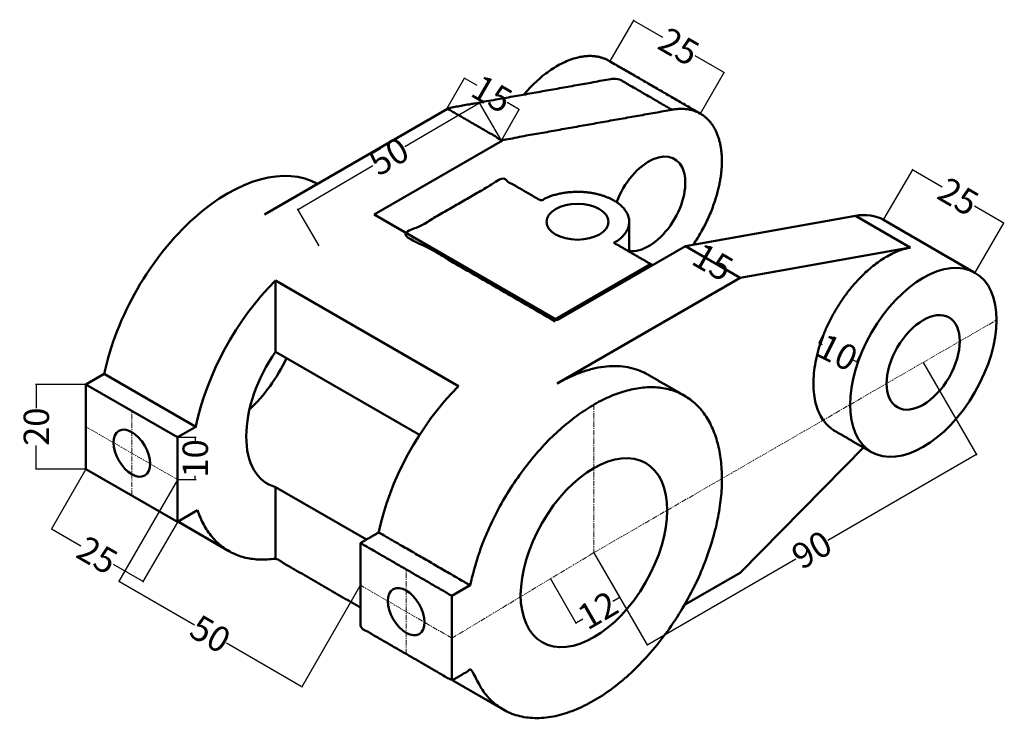
# Model space of a CAD drawing. Units: millimetres. Extents: x -15 to 218, y 4 to 169.
import ezdxf

# ---------------------------------------------------------------- set-up
doc = ezdxf.new("R2010")
doc.units = ezdxf.units.MM
doc.header["$MEASUREMENT"] = 0
doc.linetypes.add('CENTER', pattern=[2, 1.25, -0.25, 0.25, -0.25])
for name, color, linetype, lineweight in [('M-CNTR', 1, 'CENTER', 18), ('M-DIMS', 2, 'Continuous', 25), ('M-OUTL', 7, 'Continuous', 50)]:
    doc.layers.add(name, color=color, linetype=linetype, lineweight=lineweight)
doc.styles.get("Standard").update_dxf_attribs({"font": 'arial.ttf'})
doc.dimstyles.get("Standard").update_dxf_attribs({"dimtxt": 6, "dimasz": 0.18, "dimexe": 0.18, "dimexo": 0.0625, "dimgap": 0.09, "dimtad": 0, "dimtoh": 1, "dimdec": 0, "dimzin": 0, "dimdsep": 46, "dimtxsty": 'Standard', "dimcen": 0.09, "dimadec": 0, "dimazin": 0, "dimtfac": 1, "dimtdec": 0, "dimtofl": 0, "dimtmove": 0, "dimatfit": 3, "dimfxl": 1, "dimtolj": 1, "dimtzin": 0, "dimarcsym": 0})

# ---------------------------------------------------------------- blocks, each defined once
blk = doc.blocks.new('*D1')
at = {"layer": 'Defpoints', "color": 0, "transparency": 16777216}
for p in [(0.9, 82.71), (-10.85, 62.71), (0.9, 62.71)]:
    blk.add_point(p, dxfattribs=at)
at = {"layer": 'M-DIMS', "color": 0, "lineweight": -2, "transparency": 16777216}
for p, q in [((0.84, 82.71), (-11.03, 82.71)), ((-10.85, 82.53), (-10.85, 77.14)), ((-10.85, 62.89), (-10.85, 68.28)), ((0.84, 62.71), (-11.03, 62.71))]:
    blk.add_line(p, q, dxfattribs=at)
at = {"layer": 'M-DIMS', "color": 0, "transparency": 16777216}
for points in [[(-10.88, 82.53), (-10.82, 82.53), (-10.85, 82.71)], [(-10.88, 62.89), (-10.82, 62.89), (-10.85, 62.71)]]:
    blk.add_solid(points, dxfattribs=at)
at = {"layer": 'M-DIMS', "color": 0, "transparency": 16777216, "insert": (-10.85, 72.71), "char_height": 6, "attachment_point": 5, "rotation": 90}
blk.add_mtext('\\A1;20', dxfattribs=at)
blk = doc.blocks.new('*D2')
at = {"layer": 'Defpoints', "color": 0, "transparency": 16777216}
for p in [(0.9, 62.71), (22.55, 50.21), (14.4, 36.09)]:
    blk.add_point(p, dxfattribs=at)
at = {"layer": 'M-DIMS', "color": 0, "lineweight": -2, "transparency": 16777216}
for p, q in [((0.87, 62.66), (-7.34, 48.44)), ((22.52, 50.16), (14.31, 35.94)), ((-7.09, 48.5), (-0.29, 44.57)), ((14.24, 36.18), (7.44, 40.11))]:
    blk.add_line(p, q, dxfattribs=at)
at = {"layer": 'M-DIMS', "color": 0, "transparency": 16777216}
for points in [[(-7.08, 48.53), (-7.11, 48.48), (-7.25, 48.59)], [(14.26, 36.21), (14.23, 36.16), (14.4, 36.09)]]:
    blk.add_solid(points, dxfattribs=at)
at = {"layer": 'M-DIMS', "color": 0, "transparency": 16777216, "insert": (3.57, 42.34), "char_height": 6, "attachment_point": 5, "rotation": 330}
blk.add_mtext('\\A1;25', dxfattribs=at)
blk = doc.blocks.new('*D3')
at = {"layer": 'Defpoints', "color": 0, "transparency": 16777216}
for p in [(22.55, 70.21), (22.55, 60.21), (26.76, 60.21)]:
    blk.add_point(p, dxfattribs=at)
at = {"layer": 'M-DIMS', "color": 0, "lineweight": -2, "transparency": 16777216}
for p, q in [((22.62, 70.21), (26.94, 70.21)), ((26.76, 70.03), (26.76, 69.31)), ((26.76, 60.39), (26.76, 61.12)), ((22.62, 60.21), (26.94, 60.21))]:
    blk.add_line(p, q, dxfattribs=at)
at = {"layer": 'M-DIMS', "color": 0, "transparency": 16777216}
for points in [[(26.73, 70.03), (26.79, 70.03), (26.76, 70.21)], [(26.73, 60.39), (26.79, 60.39), (26.76, 60.21)]]:
    blk.add_solid(points, dxfattribs=at)
at = {"layer": 'M-DIMS', "color": 0, "transparency": 16777216, "insert": (26.76, 65.21), "char_height": 6, "attachment_point": 5, "rotation": 90}
blk.add_mtext('\\A1;10', dxfattribs=at)
blk = doc.blocks.new('*D4')
at = {"layer": 'Defpoints', "color": 0, "transparency": 16777216}
for p in [(22.55, 60.21), (8.69, 36.21), (65.85, 35.21)]:
    blk.add_point(p, dxfattribs=at)
at = {"layer": 'M-DIMS', "color": 0, "lineweight": -2, "transparency": 16777216}
for p, q in [((22.52, 60.16), (8.6, 36.05)), ((8.85, 36.12), (26.55, 25.89)), ((65.82, 35.16), (51.9, 11.05)), ((51.84, 11.3), (34.13, 21.52))]:
    blk.add_line(p, q, dxfattribs=at)
at = {"layer": 'M-DIMS', "color": 0, "transparency": 16777216}
for points in [[(8.86, 36.14), (8.83, 36.09), (8.69, 36.21)], [(51.85, 11.32), (51.82, 11.27), (51.99, 11.21)]]:
    blk.add_solid(points, dxfattribs=at)
at = {"layer": 'M-DIMS', "color": 0, "transparency": 16777216, "insert": (30.34, 23.71), "char_height": 6, "attachment_point": 5, "rotation": 330}
blk.add_mtext('\\A1;50', dxfattribs=at)
blk = doc.blocks.new('*D5')
at = {"layer": 'Defpoints', "color": 0, "transparency": 16777216}
for p in [(90.5, 155.18), (86.35, 147.99), (99.28, 140.52)]:
    blk.add_point(p, dxfattribs=at)
at = {"layer": 'M-DIMS', "color": 0, "lineweight": -2, "transparency": 16777216}
for p, q in [((86.38, 148.04), (90.59, 155.34)), ((90.66, 155.09), (93.4, 153.51)), ((103.28, 147.8), (100.54, 149.38)), ((99.32, 140.57), (103.53, 147.87))]:
    blk.add_line(p, q, dxfattribs=at)
at = {"layer": 'M-DIMS', "color": 0, "transparency": 16777216}
for points in [[(90.67, 155.12), (90.64, 155.07), (90.5, 155.18)], [(103.3, 147.83), (103.27, 147.78), (103.44, 147.71)]]:
    blk.add_solid(points, dxfattribs=at)
at = {"layer": 'M-DIMS', "color": 0, "transparency": 16777216, "insert": (96.97, 151.45), "char_height": 6, "attachment_point": 5, "rotation": 330}
blk.add_mtext('\\A1;15', dxfattribs=at)
blk = doc.blocks.new('*D6')
at = {"layer": 'Defpoints', "color": 0, "transparency": 16777216}
for p in [(94.05, 149.29), (99.13, 140.61), (56.14, 115.43)]:
    blk.add_point(p, dxfattribs=at)
at = {"layer": 'M-DIMS', "color": 0, "lineweight": -2, "transparency": 16777216}
for p, q in [((93.89, 149.2), (76.33, 138.91)), ((99.1, 140.66), (93.96, 149.45)), ((51.21, 124.2), (68.77, 134.49)), ((56.11, 115.48), (50.96, 124.27))]:
    blk.add_line(p, q, dxfattribs=at)
at = {"layer": 'M-DIMS', "color": 0, "transparency": 16777216}
for points in [[(93.88, 149.23), (93.91, 149.17), (94.05, 149.29)], [(51.19, 124.23), (51.22, 124.18), (51.05, 124.11)]]:
    blk.add_solid(points, dxfattribs=at)
at = {"layer": 'M-DIMS', "color": 0, "transparency": 16777216, "insert": (72.55, 136.7), "char_height": 6, "attachment_point": 5, "rotation": 30.3547}
blk.add_mtext('\\A1;50', dxfattribs=at)
blk = doc.blocks.new('*D7')
at = {"layer": 'Defpoints', "color": 0, "transparency": 16777216}
for p in [(199.03, 87.93), (211.62, 66.13), (121.09, 42.93)]:
    blk.add_point(p, dxfattribs=at)
at = {"layer": 'M-DIMS', "color": 0, "lineweight": -2, "transparency": 16777216}
for p, q in [((199.06, 87.88), (211.71, 65.97)), ((211.46, 66.04), (176.44, 45.82)), ((121.12, 42.88), (133.77, 20.97)), ((133.83, 21.22), (168.86, 41.44))]:
    blk.add_line(p, q, dxfattribs=at)
at = {"layer": 'M-DIMS', "color": 0, "transparency": 16777216}
for points in [[(211.45, 66.06), (211.48, 66.01), (211.62, 66.13)], [(133.82, 21.24), (133.85, 21.19), (133.68, 21.13)]]:
    blk.add_solid(points, dxfattribs=at)
at = {"layer": 'M-DIMS', "color": 0, "transparency": 16777216, "insert": (172.65, 43.63), "char_height": 6, "attachment_point": 5, "rotation": 30}
blk.add_mtext('\\A1;90', dxfattribs=at)
blk = doc.blocks.new('*D8')
at = {"layer": 'Defpoints', "color": 0, "transparency": 16777216}
for p in [(121.09, 42.93), (110.7, 36.93), (127.21, 32.32)]:
    blk.add_point(p, dxfattribs=at)
at = {"layer": 'M-DIMS', "color": 0, "lineweight": -2, "transparency": 16777216}
for p, q in [((121.12, 42.88), (127.3, 32.17)), ((110.73, 36.88), (116.91, 26.17)), ((127.06, 32.23), (125.55, 31.36)), ((116.98, 26.41), (118.49, 27.29))]:
    blk.add_line(p, q, dxfattribs=at)
at = {"layer": 'M-DIMS', "color": 0, "transparency": 16777216}
for points in [[(127.04, 32.26), (127.07, 32.21), (127.21, 32.32)], [(116.96, 26.44), (116.99, 26.39), (116.82, 26.32)]]:
    blk.add_solid(points, dxfattribs=at)
at = {"layer": 'M-DIMS', "color": 0, "transparency": 16777216, "insert": (122.02, 29.32), "char_height": 6, "attachment_point": 5, "rotation": 30}
blk.add_mtext('\\A1;12', dxfattribs=at)
blk = doc.blocks.new('*D9')
at = {"layer": 'Defpoints', "color": 0, "transparency": 16777216}
for p in [(196.56, 133.48), (189.7, 121.77), (211.28, 109.14)]:
    blk.add_point(p, dxfattribs=at)
at = {"layer": 'M-DIMS', "color": 0, "lineweight": -2, "transparency": 16777216}
for p, q in [((189.74, 121.83), (196.65, 133.63)), ((196.71, 133.39), (203.49, 129.42)), ((217.98, 120.94), (211.19, 124.91)), ((211.31, 109.2), (218.22, 121))]:
    blk.add_line(p, q, dxfattribs=at)
at = {"layer": 'M-DIMS', "color": 0, "transparency": 16777216}
for points in [[(196.73, 133.41), (196.7, 133.36), (196.56, 133.48)], [(217.99, 120.97), (217.96, 120.91), (218.13, 120.85)]]:
    blk.add_solid(points, dxfattribs=at)
at = {"layer": 'M-DIMS', "color": 0, "transparency": 16777216, "insert": (207.34, 127.16), "char_height": 6, "attachment_point": 5, "rotation": 329.6597}
blk.add_mtext('\\A1;25', dxfattribs=at)
blk = doc.blocks.new('*D10')
at = {"layer": 'Defpoints', "color": 0, "transparency": 16777216}
for p in [(176.96, 97.84), (185.88, 93.36), (174.3, 92.55)]:
    blk.add_point(p, dxfattribs=at)
at = {"layer": 'M-DIMS', "color": 0, "lineweight": -2, "transparency": 16777216}
for p, q in [((176.93, 97.79), (174.22, 92.39)), ((185.86, 93.3), (183.15, 87.91)), ((174.46, 92.47), (175.1, 92.15)), ((183.07, 88.15), (182.42, 88.47))]:
    blk.add_line(p, q, dxfattribs=at)
at = {"layer": 'M-DIMS', "color": 0, "transparency": 16777216}
for points in [[(174.48, 92.5), (174.45, 92.44), (174.3, 92.55)], [(183.08, 88.17), (183.05, 88.12), (183.23, 88.07)]]:
    blk.add_solid(points, dxfattribs=at)
at = {"layer": 'M-DIMS', "color": 0, "transparency": 16777216, "insert": (178.76, 90.31), "char_height": 6, "attachment_point": 5, "rotation": 333.326}
blk.add_mtext('\\A1;10', dxfattribs=at)
blk = doc.blocks.new('*D11')
at = {"layer": 'Defpoints', "color": 0, "transparency": 16777216}
for p in [(142.74, 115.43), (155.73, 107.93), (155.73, 107.93)]:
    blk.add_point(p, dxfattribs=at)
at = {"layer": 'M-DIMS', "color": 0, "lineweight": -2, "transparency": 16777216}
for p, q in [((142.77, 115.48), (142.83, 115.59)), ((142.9, 115.34), (145.66, 113.74)), ((155.58, 108.02), (152.81, 109.62)), ((155.76, 107.98), (155.82, 108.09))]:
    blk.add_line(p, q, dxfattribs=at)
at = {"layer": 'M-DIMS', "color": 0, "transparency": 16777216}
for points in [[(142.91, 115.37), (142.88, 115.31), (142.74, 115.43)], [(155.59, 108.05), (155.56, 107.99), (155.73, 107.93)]]:
    blk.add_solid(points, dxfattribs=at)
at = {"layer": 'M-DIMS', "color": 0, "transparency": 16777216, "insert": (149.24, 111.68), "char_height": 6, "attachment_point": 5, "rotation": 330}
blk.add_mtext('\\A1;15', dxfattribs=at)
blk = doc.blocks.new('*D12')
at = {"layer": 'Defpoints', "color": 0, "transparency": 16777216}
for p in [(130.5, 168.83), (124.9, 159.12), (146.31, 146.76)]:
    blk.add_point(p, dxfattribs=at)
at = {"layer": 'M-DIMS', "color": 0, "lineweight": -2, "transparency": 16777216}
for p, q in [((124.93, 159.17), (130.59, 168.99)), ((130.66, 168.74), (137.35, 164.88)), ((151.76, 156.56), (145.07, 160.42)), ((146.34, 146.81), (152, 156.63))]:
    blk.add_line(p, q, dxfattribs=at)
at = {"layer": 'M-DIMS', "color": 0, "transparency": 16777216}
for points in [[(130.67, 168.77), (130.64, 168.72), (130.5, 168.83)], [(151.77, 156.59), (151.74, 156.53), (151.91, 156.47)]]:
    blk.add_solid(points, dxfattribs=at)
at = {"layer": 'M-DIMS', "color": 0, "transparency": 16777216, "insert": (141.21, 162.65), "char_height": 6, "attachment_point": 5, "rotation": 330}
blk.add_mtext('\\A1;25', dxfattribs=at)

msp = doc.modelspace()

# ---------------------------------------------------------------- linework, layer by layer
at = {"layer": 'M-CNTR'}
for p, q in [((11.73, 56.46), (11.73, 76.46)), ((0.9, 72.71), (22.55, 60.21)), ((76.68, 18.96), (76.68, 38.96))]:
    msp.add_line(p, q, dxfattribs=at)
for points in [[(121.09, 77.93), (121.09, 42.93), (216.35, 97.93)], [(121.09, 42.93), (87.5, 22.71), (65.85, 35.21)]]:
    msp.add_lwpolyline(points, dxfattribs=at)
at = {"layer": 'M-OUTL'}
for p, q in [((43.15, 122.93), (86.45, 147.93)), ((69.13, 122.93), (99.44, 140.43)), ((112.43, 97.93), (69.13, 122.93)), ((129.45, 121.2), (129.45, 114.13)), ((195.97, 115.09), (182.98, 122.59)), ((211.28, 109.15), (189.63, 121.65)), ((112.43, 97.93), (142.74, 115.43)), ((155.73, 107.93), (195.97, 115.09)), ((112, 98.18), (134.51, 111.18)), ((89.05, 82.31), (45.74, 107.31)), ((45.74, 90.43), (45.74, 107.31)), ((112.43, 82.93), (155.73, 107.93)), ((79.81, 70.77), (45.74, 90.43)), ((34.7, 43.31), (22.8, 50.18)), ((99.66, 5.81), (87.75, 12.68))]:
    msp.add_line(p, q, dxfattribs=at)
for points in [[(155.73, 107.93), (142.74, 115.43), (183.04, 122.6)], [(22.55, 70.21), (0.9, 82.71), (5.23, 85.21), (26.88, 72.71), (22.55, 70.21), (22.55, 50.21), (0.9, 62.71), (0.9, 82.71)], [(142.52, 30.56), (155.73, 38.18), (185.1, 68)], [(45.75, 41.55), (45.75, 58.43), (67.25, 46.02)], [(87.5, 12.71), (87.5, 32.71), (91.83, 35.21)]]:
    msp.add_lwpolyline(points, dxfattribs=at)
msp.add_lwpolyline([(27.31, 52.96), (22.55, 50.21)], close=True, dxfattribs=at)
for centre, major_axis, start_param, end_param in [((134.08, 125.43), (-6.12, -10.61), 6.504834, 11.282198), ((34.49, 92.93), (-21.43, -37.12), 9.434983, 11.515891), ((177.38, 100.43), (12.25, 21.21), 0, 0.456461), ((56.14, 80.43), (21.43, 37.12), 1.135355, 2.09613), ((56.14, 80.43), (-12.25, -21.21), 4.570492, 6.425082), ((34.49, 92.93), (-12.25, -21.21), 7.367287, 7.995879), ((99.44, 55.43), (21.43, 37.12), 1.135355, 2.09613)]:
    msp.add_ellipse(centre, major_axis=major_axis, ratio=0.57735, start_param=start_param, end_param=end_param, dxfattribs=at)
for centre, major_axis in [((117.21, 121.2), (-7.35, 0)), ((199.03, 87.93), (-12.25, -21.21)), ((199.03, 87.93), (-6.12, -10.61)), ((11.73, 66.46), (3.06, -5.3)), ((121.09, 42.93), (-12.25, -21.21)), ((76.68, 28.96), (3.06, -5.3))]:
    msp.add_ellipse(centre, major_axis=major_axis, ratio=0.57735, dxfattribs=at)
for points, weights, knots in [([(146.31, 146.76), (135.48, 153.01), (124.66, 159.26), (115.72, 164.42), (104.49, 151.26)], [1, 1, 1, 0.807904624626, 1], [0, 0, 0, 1, 1, 2.260417, 2.260417, 2.260417]), ([(144.69, 115.9), (152.87, 127.96), (151.14, 138.75), (149.4, 149.54), (139.59, 147.69), (133.09, 151.44), (126.6, 155.19), (106.45, 151.61), (86.29, 148.02), (92.79, 144.27), (99.28, 140.52), (119.44, 144.11), (139.59, 147.69)], [1, 0.858253514153, 1, 0.858253514153, 1, 1, 1, 1, 1, 1, 1, 1, 1], [0, 0, 0, 1.077879, 1.077879, 2.155757, 2.155757, 3.155757, 3.155757, 4.155757, 4.155757, 5.155757, 5.155757, 6.155757, 6.155757, 6.155757]), ([(134.97, 110.94), (130.42, 113.57), (125.87, 116.2), (134.53, 121.2), (125.87, 126.2), (117.21, 131.2), (108.55, 126.2), (103.99, 128.83), (99.44, 131.46), (87.92, 124.81), (76.4, 118.16), (94.17, 107.9), (111.93, 97.64)], [1, 1, 1, 0.707106781187, 1, 0.707106781187, 1, 1, 1, 1, 1, 1, 1], [0, 0, 0, 1, 1, 2.570796, 2.570796, 4.141593, 4.141593, 5.141593, 5.141593, 6.141593, 6.141593, 7.141593, 7.141593, 7.141593]), ([(196.03, 115.1), (183.01, 112.78), (175.69, 95.06), (168.38, 77.35), (178.13, 71.72), (182.46, 69.22), (186.79, 66.72)], [1, 0.782385478434, 1, 0.782385478434, 1, 1, 1], [0, 0, 0, 1.344619, 1.344619, 2.689238, 2.689238, 3.689238, 3.689238, 3.689238]), ([(142.52, 80.05), (138.19, 82.55), (133.86, 85.05), (124.99, 90.18), (112.43, 82.93)], [1, 1, 1, 0.923879532511, 1], [0, 0, 0, 1, 1, 1.785398, 1.785398, 1.785398]), ([(65.85, 45.21), (65.85, 35.21), (65.85, 25.21), (76.68, 18.96), (87.5, 12.71), (89.89, 14.09), (92.27, 15.46), (100.37, -8.64), (126.21, 11.39), (152.04, 31.41), (151.39, 61.29), (150.74, 91.17), (124.72, 79.78), (98.7, 68.38), (91.84, 35.21), (91.84, 35.21), (91.83, 35.21), (81.01, 41.46), (70.18, 47.71), (68.02, 46.46), (65.85, 45.21), (76.68, 38.96), (87.5, 32.71)], [1, 1, 1, 1, 1, 1, 1, 0.756436998466, 1, 0.756436998466, 1, 0.756436998466, 1, 0.756436998466, 1, 1, 1, 1, 1, 1, 1, 1, 1], [0, 0, 0, 1, 1, 2, 2, 3, 3, 4.425896, 4.425896, 5.851792, 5.851792, 7.277688, 7.277688, 8.703584, 8.703584, 9.703584, 9.703584, 10.703584, 10.703584, 11.703584, 11.703584, 12.703584, 12.703584, 12.703584]), ([(27.31, 52.96), (31.88, 39.39), (45.75, 41.55), (55.8, 35.75), (65.85, 29.94)], [1, 0.899068166052, 1, 1, 1], [0, 0, 0, 0.90632, 0.90632, 1.90632, 1.90632, 1.90632])]:
    msp.add_rational_spline(points, weights, degree=2, knots=knots, dxfattribs=at)

# ---------------------------------------------------------------- dimensions: what is measured, and where the dimension line sits
at = {"layer": 'M-DIMS'}
for p1, p2, distance, picture, middle in [((146.31, 146.76), (124.9, 159.12), -11.21, '*D12', (141.21, 162.65)), ((99.28, 140.52), (86.35, 147.99), -8.31, '*D5', (96.97, 151.45)), ((56.14, 115.43), (99.13, 140.61), 10.06, '*D6', (72.55, 136.7)), ((211.28, 109.14), (189.7, 121.77), -13.56, '*D9', (207.34, 127.16)), ((142.74, 115.43), (155.73, 107.93), 0, '*D11', (149.24, 111.68)), ((185.88, 93.36), (176.96, 97.84), 5.92, '*D10', (178.76, 90.31)), ((121.09, 42.93), (199.03, 87.93), -25.17, '*D7', (172.65, 43.63)), ((0.9, 82.71), (0.9, 62.71), -11.75, '*D1', (-10.85, 72.71)), ((22.55, 70.21), (22.55, 60.21), 4.2, '*D3', (26.76, 65.21)), ((0.9, 62.71), (22.55, 50.21), -16.31, '*D2', (3.57, 42.34)), ((65.85, 35.21), (22.55, 60.21), 27.72, '*D4', (30.34, 23.71)), ((110.7, 36.93), (121.09, 42.93), -12.25, '*D8', (122.02, 29.32))]:
    dim = msp.add_aligned_dim(p1=p1, p2=p2, distance=distance, dimstyle='Standard', override={"dimclrd": 0, "dimclre": 0, "dimclrt": 0}, dxfattribs=at)
    dim.commit()
    dim.dimension.update_dxf_attribs({"geometry": picture, "text_midpoint": middle})

doc.saveas('drawing.dxf')
